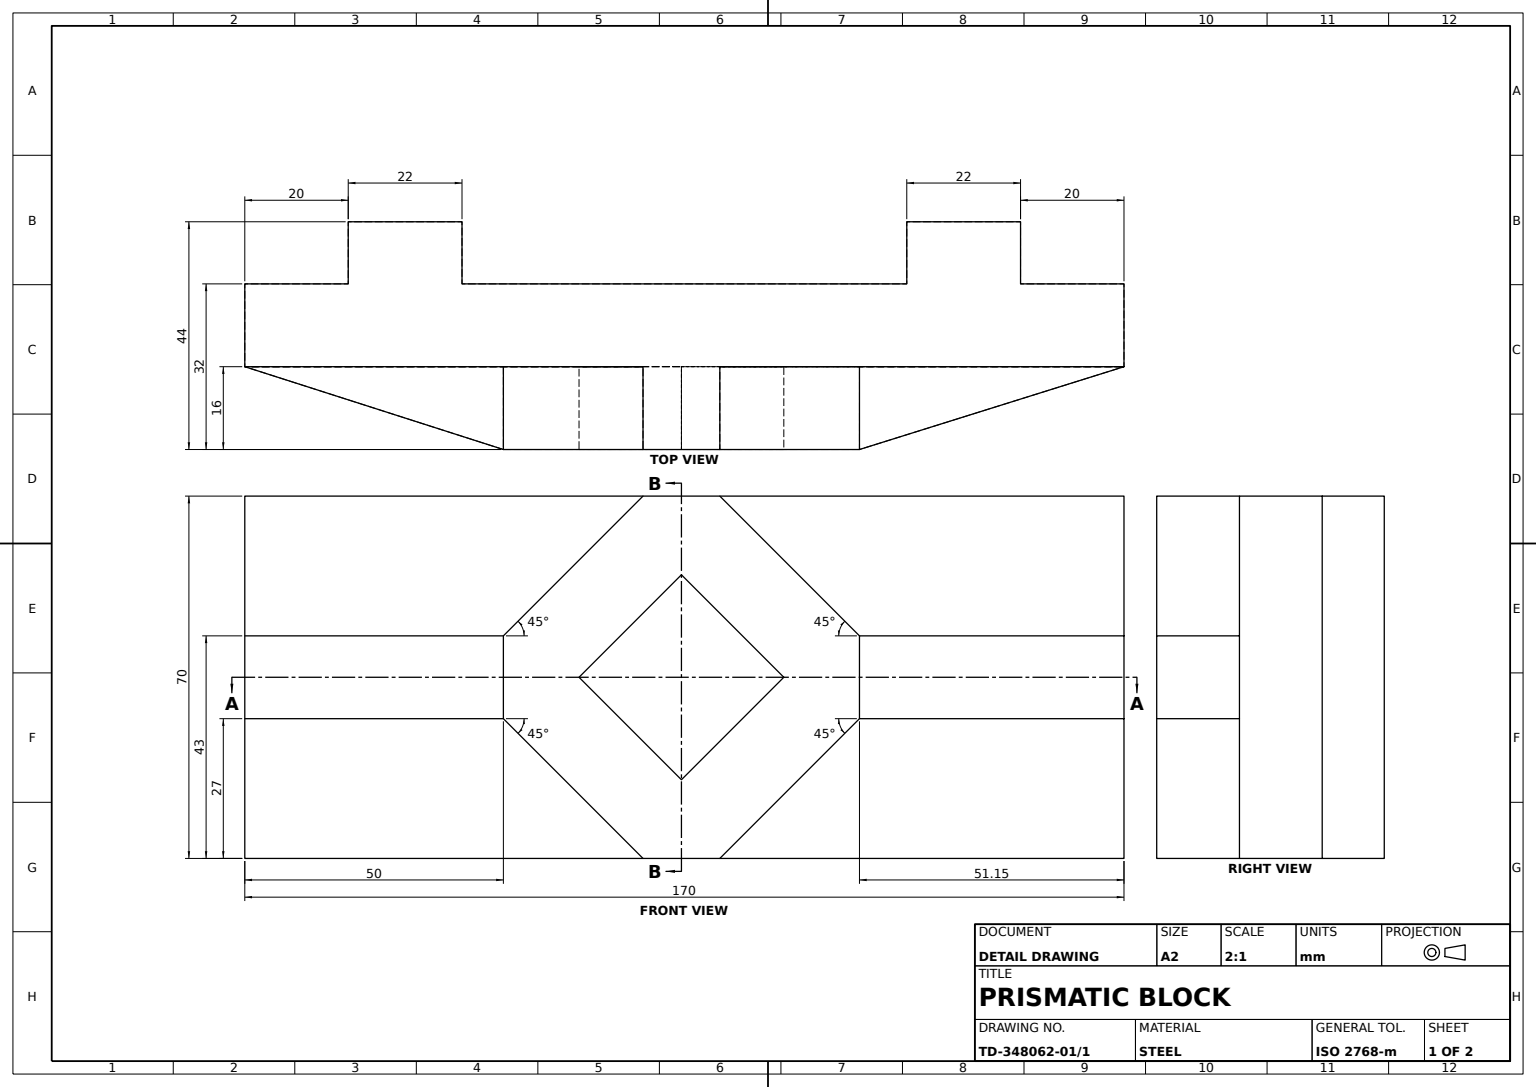
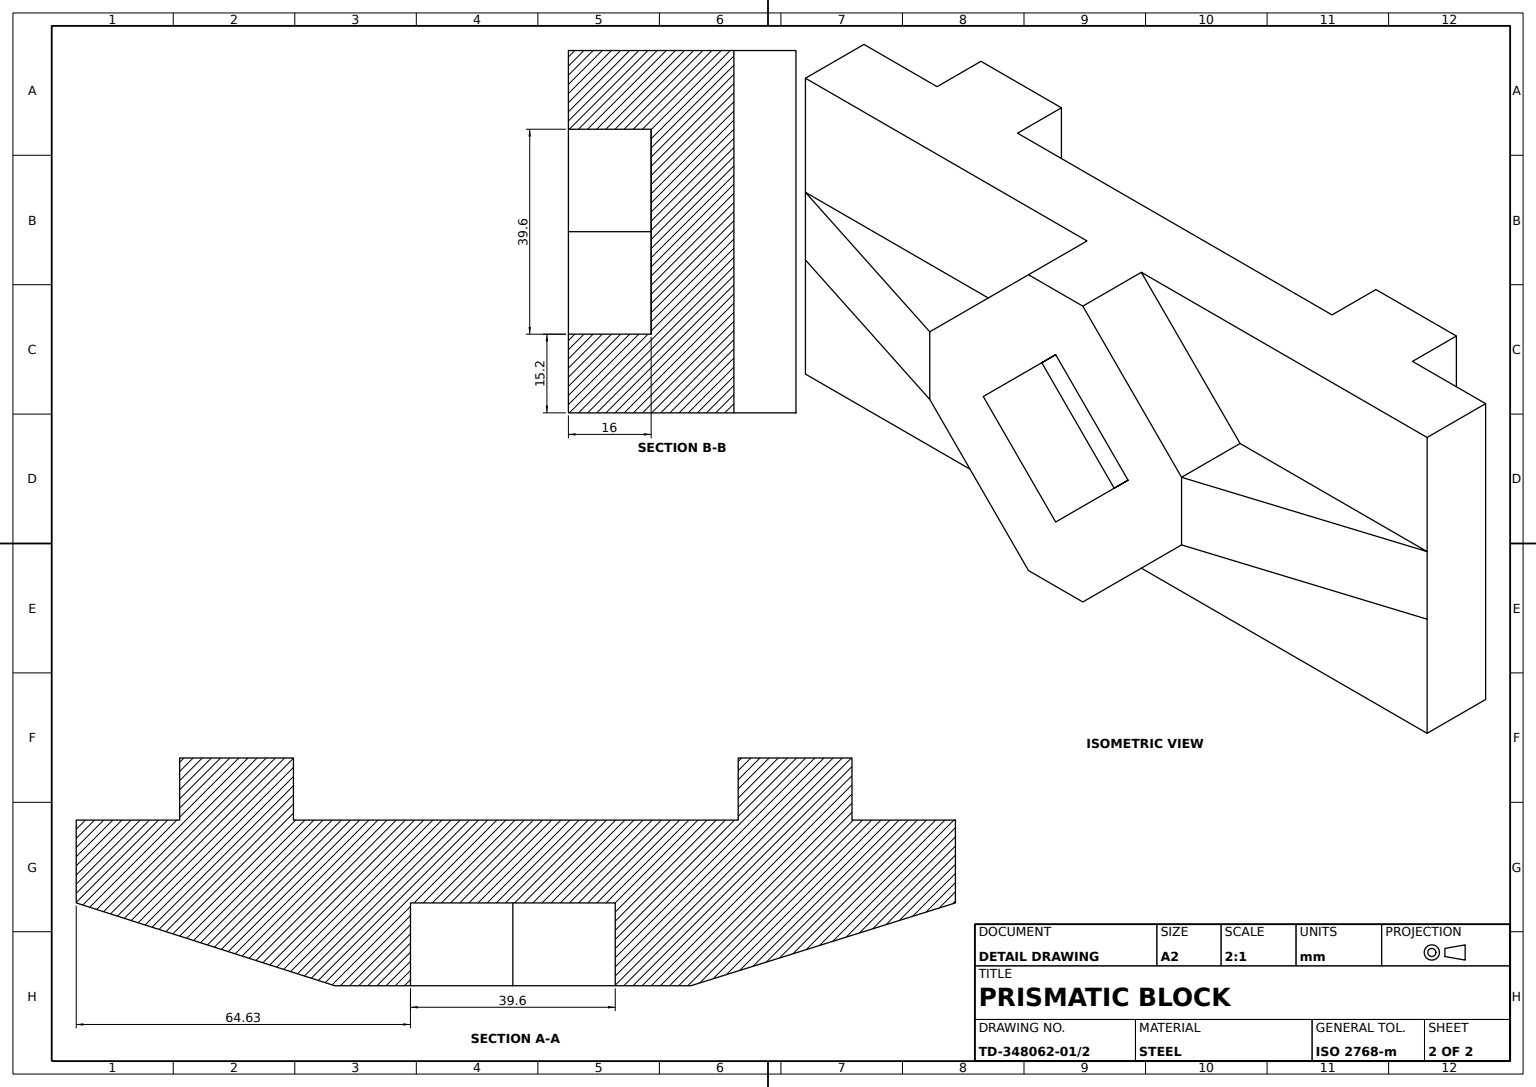
SolidWorks part; units mm, degrees
material "Plain Carbon Steel"
ref_plane "Front Plane" through (0, 0, 0) normal (0, 0, 1) x (1, 0, 0)
ref_plane "Top Plane" through (0, 0, 0) normal (0, 1, 0) x (1, 0, 0)
ref_plane "Right Plane" through (0, 0, 0) normal (1, 0, 0) x (0, 0, -1)
sketch "Base Plate Sketch" plane through (0, 0, 0) normal (0, 0, 1) x (1, 0, 0)
  line L0 (0, 0) -> (170, 0)
  line L1 (170, 0) -> (170, 70)
  line L2 (170, 70) -> (0, 70)
  line L3 (0, 70) -> (0, 0)
  dimension "D1" = 170
  dimension "D2" = 70
extrude "Base Plate 16mm" add sketch "Base Plate Sketch" along normal blind 16
sketch "Center Boss Sketch" plane through (0, 0, 16) normal (0, 0, 1) x (1, 0, 0)
  line L0 (0, 70) -> (0, 0) construction
  line L1 (170, 70) -> (0, 70) construction
  line L2 (0, 0) -> (170, 0) construction
  line L6 (85, 70) -> (77, 70)
  line L7 (77, 70) -> (91.8528, 70)
  line L13 (85, 0) -> (91.8528, 0)
  line L14 (91.8528, 0) -> (77, 0)
  line L15 (50, 35) -> (50, 43)
  line L16 (50, 43) -> (50, 27)
  line L17 (118.8528, 35) -> (118.8528, 43)
  line L18 (118.8528, 43) -> (118.8528, 27)
  line L19 (91.8528, 70) -> (118.8528, 43)
  line L20 (50, 27) -> (77, 0)
  line L21 (77, 70) -> (50, 43)
  line L22 (118.8528, 27) -> (91.8528, 0)
  line M6 (0, 0) -> (170, 0)
  line M8 (170, 70) -> (0, 70)
  dimension "D1" = 60
  dimension "D2" = 60
  dimension "D3" = 77
extrude "Center Boss 60x60" add sketch "Center Boss Sketch" along normal blind 16 contours L22 L18 L17 L19 L21 L15 L16 L20 M8 M6
sketch "Center Pocket Sketch" plane through (0, 0, 32) normal (0, 0, 1) x (1, 0, 0)
  line L0 (118.8528, 43) -> (118.8528, 27) construction
  line L1 (91.8528, 70) -> (77, 70) construction
  line L7 (84.4264, 15.201) -> (104.2254, 35)
  line L8 (104.2254, 35) -> (84.4264, 54.799)
  line L9 (84.4264, 54.799) -> (64.6274, 35)
  line L10 (84.4264, 15.201) -> (64.6274, 35)
  dimension "D1" = 28
  dimension "D2" = 14.6274
  dimension "D3" = 15.201
extrude "Center Pocket 28" cut sketch "Center Pocket Sketch" against normal blind 16
sketch "Left Wedge Sketch" plane through (0, 0, 0) normal (0, -1, 0) x (1, 0, 0)
  line L0 (118.8528, 32) -> (118.8528, 16)
  line L1 (118.8528, 16) -> (170, 16)
  line L2 (170, 16) -> (118.8528, 32)
extrude "Left Wedge Boss" add sketch "Left Wedge Sketch" against normal blind 43
sketch "Left Wedge Cut Sketch" plane through (0, 0, 0) normal (0, -1, 0) x (1, 0, 0)
  line L0 (118.8528, 32) -> (118.8528, 16)
  line L1 (118.8528, 16) -> (170, 16)
  line L2 (170, 16) -> (118.8528, 32)
extrude "Left Wedge Cut" cut sketch "Left Wedge Cut Sketch" against normal blind 27
sketch "Right Wedge Sketch" plane through (0, 0, 0) normal (0, -1, 0) x (1, 0, 0)
  line L0 (50, 32) -> (50, 16)
  line L1 (50, 16) -> (0, 16)
  line L2 (0, 16) -> (50, 32)
extrude "Right Wedge Boss" add sketch "Right Wedge Sketch" against normal blind 43
sketch "Right Wedge Cut Sketch" plane through (0, 0, 0) normal (0, -1, 0) x (1, 0, 0)
  line L0 (50, 32) -> (50, 16)
  line L1 (50, 16) -> (0, 16)
  line L2 (0, 16) -> (50, 32)
extrude "Right Wedge Cut" cut sketch "Right Wedge Cut Sketch" against normal blind 27
sketch "Top Rail Sketch" plane through (0, 0, 0) normal (0, -1, 0) x (1, 0, 0)
  line L0 (0, 16) -> (0, 0) construction
  line L1 (0, 0) -> (170, 0) construction
  line L2 (20, 0) -> (20, -12)
  line L3 (20, -12) -> (42, -12)
  line L4 (42, -12) -> (42, 0)
  line L5 (42, 0) -> (20, 0)
  line L6 (150, 0) -> (150, -12)
  line L7 (150, -12) -> (128, -12)
  line L8 (128, -12) -> (128, 0)
  line L9 (128, 0) -> (150, 0)
  dimension "D1" = 20
  dimension "D2" = 42
  dimension "D3" = 128
  dimension "D4" = 12
extrude "Top Rail with Tabs" add sketch "Top Rail Sketch" against normal blind 70
